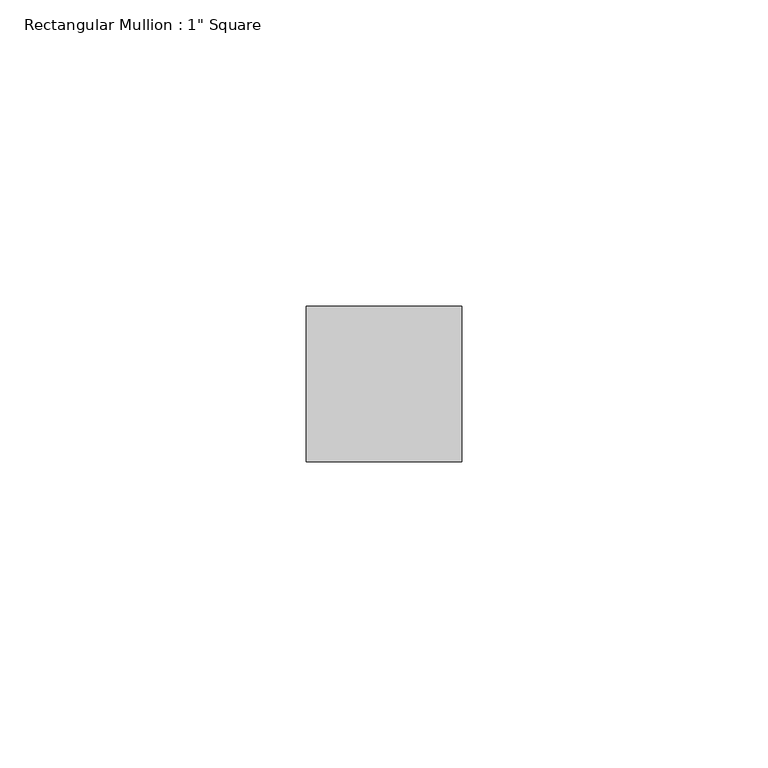
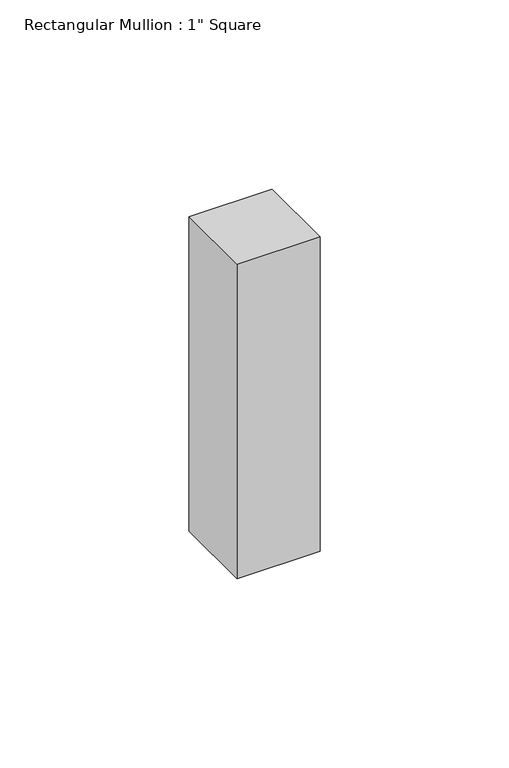
"""IFC4 building model written with IfcOpenShell, lengths in millimetres: member geometry."""

from ifc_helpers import new_model, si_unit, frame, origin, place, context, project, spatial, polyline, outline, extrude, source, transform, mapped, element, save


def member_d2c643f7(model_context):
    return source(origin(), model_context, "Body", "SweptSolid", [
        extrude(outline(polyline([(0.0, 12.7), (0.0, -12.7), (-25.4, -12.7), (-25.4, 12.7), (0.0, 12.7)])), frame((0.0, 0.0, -101.6), z_axis=(0.0, 0.0, 1.0), x_axis=(1.0, 0.0, 0.0)), (0.0, 0.0, 1.0), 101.6),
    ])


if __name__ == "__main__":
    model = new_model("IFC4")
    model_context = context("Model", 3, world=origin())
    ifc_project = project(units=[si_unit("LENGTHUNIT", "METRE", prefix="MILLI")], contexts=[model_context])
    site = spatial("IfcSite", under=ifc_project)
    building = spatial("IfcBuilding", under=site)
    placement = place(None, origin())
    member_shape = member_d2c643f7(model_context)
    element("IfcMember", 1, ObjectType="Rectangular Mullion : 1\" Square", at=placement, inside=building, context=model_context, shape_type="MappedRepresentation", body=[
        mapped(member_shape, transform((0.0, 0.0, 0.0), x_axis=(1.0, 0.0, 0.0), y_axis=(0.0, 1.0, 0.0), z_axis=(0.0, 0.0, 1.0))),
    ])
    save(model, "model.ifc")

# Revit data of these elements
# Type "Rectangular Mullion : 1\" Square"
#   built-in parameter 1007304 = 0.0833333 (stored number, unit not read)
#   built-in parameter 1007301 = 0.0416667 (stored number, unit not read)
#   built-in parameter 1007300 = 0.0416667 (stored number, unit not read)
# Element 1 (IfcMember, "Rectangular Mullion : 1\" Square")
#   Materials on its faces: "black"
# Materials
#   "black": class "Generic", colour RGB 120 120 120, transparency 0, Cost = 0
